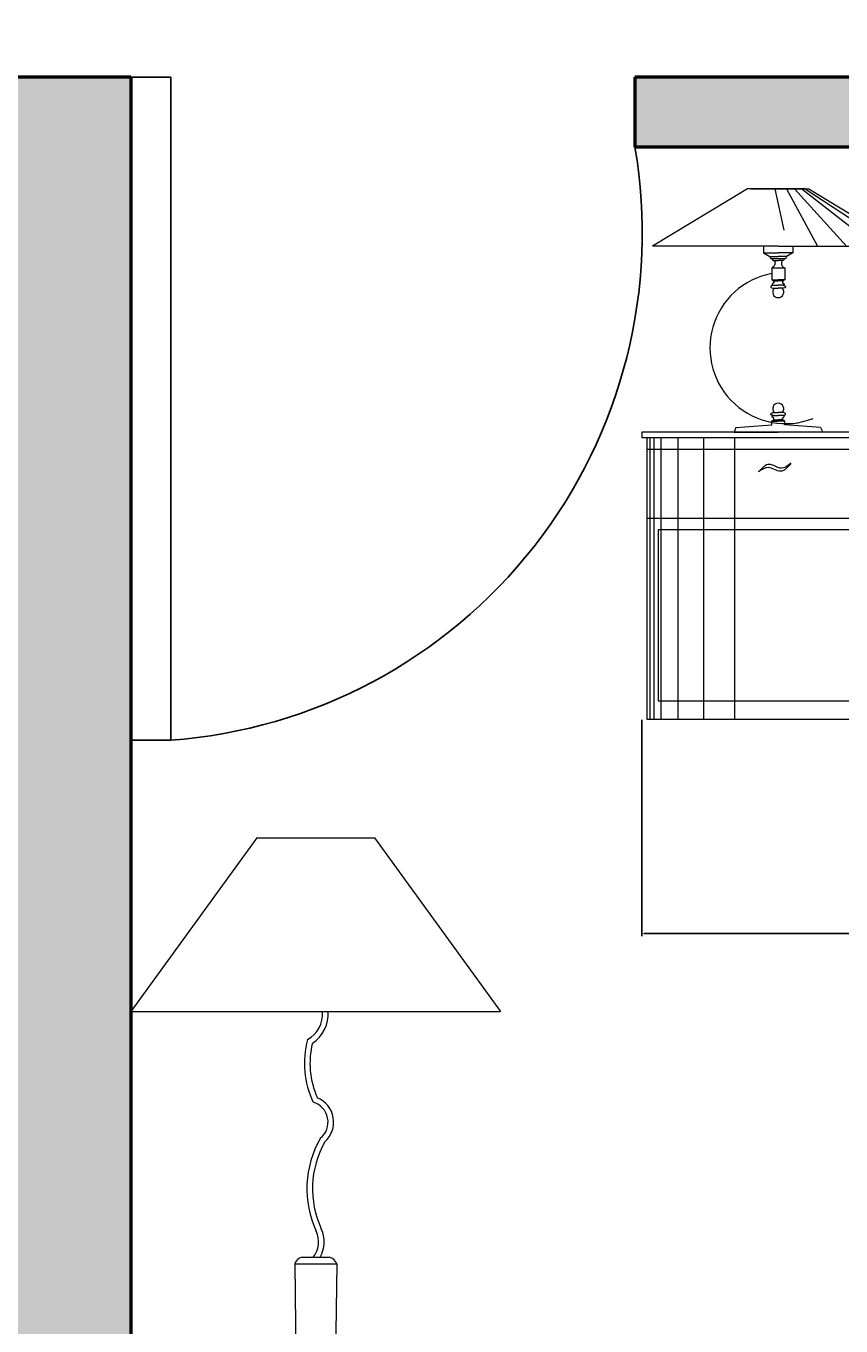
# Model space of a CAD drawing. Units: inches. Extents: x 1771 to 3025, y 319 to 889.
# Tile 3 of 35: x 1939 to 1997, y 527 to 620. Entities that reach past the tile are written whole.
import ezdxf

# ---------------------------------------------------------------- set-up
doc = ezdxf.new("R2010")
doc.units = ezdxf.units.IN
doc.header["$MEASUREMENT"] = 0
for name, color, linetype, lineweight in [('A-ANNO-DIMS', 2, 'Continuous', 18), ('A-DOOR', 4, 'Continuous', 25), ('A-FURN', 8, 'Continuous', 18), ('A-WALL', 7, 'Continuous', 50), ('A-WALL-PATT', 254, 'Continuous', 13)]:
    doc.layers.add(name, color=color, linetype=linetype, lineweight=lineweight)
doc.styles.get("Standard").update_dxf_attribs({"font": 'arial.ttf'})
doc.dimstyles.get("Standard").update_dxf_attribs({"dimtxt": 0.18, "dimasz": 0.18, "dimexe": 0.18, "dimexo": 0.0625, "dimgap": 0.09, "dimtad": 0, "dimtih": 1, "dimtoh": 1, "dimdec": 4, "dimzin": 0, "dimdsep": 46, "dimtxsty": 'Standard', "dimcen": 0.09, "dimadec": 0, "dimazin": 0, "dimtfac": 1, "dimtdec": 4, "dimtofl": 0, "dimtmove": 0, "dimatfit": 3, "dimfxl": 1, "dimtolj": 1, "dimtzin": 0, "dimarcsym": 0})

# ---------------------------------------------------------------- blocks, each defined once
blk = doc.blocks.new('A$C3908634B')
for p, q in [((184.3, 923.4), (19, 823.1)), ((237.5, 923.4), (184.3, 923.4)), ((190.2, 923.4), (237.5, 923.4)), ((231.9, 923.4), (247.3, 851.1)), ((284.7, 923.4), (237.5, 923.4)), ((237.5, 923.4), (290.6, 923.4)), ((251.7, 923.4), (305.7, 823.1)), ((266, 923.4), (356.4, 823.1)), ((278.7, 923.4), (406.8, 823.1)), ((284.7, 923.4), (436.3, 823.1)), ((290.6, 923.4), (456, 823.1)), ((237.5, 823.1), (19, 823.1)), ((212, 823.1), (212, 811.7)), ((237.5, 823.1), (456, 823.1)), ((263, 823.1), (263, 811.7)), ((212, 811.7), (223, 805.4)), ((212, 811.7), (237.5, 811.7)), ((223, 805.4), (224.6, 801.4)), ((223, 805.4), (237.5, 805.4)), ((250.4, 801.4), (224.6, 801.4)), ((226.9, 801.4), (228.3, 798.3)), ((228.3, 798.3), (237.5, 798.3)), ((228.3, 798.3), (231.3, 797.6)), ((231.3, 797.6), (232, 794.9)), ((231.6, 792.6), (231.5, 791.9)), ((231.9, 793.9), (231.6, 792.6)), ((232, 794.9), (231.9, 793.9)), ((263, 811.7), (237.5, 811.7)), ((252, 805.4), (237.5, 805.4)), ((246.7, 798.3), (237.5, 798.3)), ((243.7, 797.6), (243, 794.9)), ((243, 794.9), (243.1, 793.9)), ((243.1, 793.9), (243.4, 792.6)), ((243.4, 792.6), (243.4, 791.9)), ((246.7, 798.3), (243.7, 797.6)), ((248.1, 801.4), (246.7, 798.3)), ((252, 805.4), (250.4, 801.4)), ((263, 811.7), (252, 805.4)), ((227.8, 786.4), (226.2, 785.6)), ((226.2, 785.6), (226.2, 765)), ((226.2, 785.6), (248.8, 785.6)), ((230.2, 788), (227.8, 786.4)), ((231.1, 790.5), (230.2, 788)), ((231.5, 791.1), (231.1, 790.5)), ((231.5, 791.9), (231.5, 791.1)), ((243.4, 791.9), (243.4, 791.1)), ((243.4, 791.1), (243.9, 790.5)), ((243.9, 790.5), (244.8, 788)), ((244.8, 788), (247.2, 786.4)), ((247.2, 786.4), (248.8, 785.6)), ((248.8, 785.6), (248.8, 765)), ((224.8, 753.5), (224.7, 752.9)), ((224.7, 752.9), (224.8, 752.1)), ((225.3, 753.9), (224.8, 753.5)), ((224.8, 752.1), (225.2, 751.4)), ((225.2, 751.4), (225.6, 750.9)), ((225.7, 754.3), (225.3, 753.9)), ((225.6, 750.9), (228.1, 750.2)), ((226.3, 754.6), (225.7, 754.3)), ((226.2, 765), (227.6, 764.2)), ((226.2, 765), (237.5, 765)), ((227, 754.7), (226.3, 754.6)), ((227.9, 754.7), (227, 754.7)), ((227.4, 757.9), (227.1, 757.2)), ((227.1, 757.2), (227.3, 756.6)), ((227.3, 756.6), (227.8, 755.9)), ((227.7, 758.5), (227.4, 757.9)), ((227.6, 764.2), (228.5, 763.3)), ((228.6, 758.7), (227.7, 758.5)), ((227.8, 755.9), (228.9, 755.2)), ((228.9, 755.2), (227.9, 754.7)), ((228.1, 750.2), (229.9, 750)), ((228.5, 763.3), (229.4, 762.5)), ((228.5, 763.3), (237.5, 763.3)), ((229.4, 759.1), (228.6, 758.7)), ((228.9, 755.2), (237.5, 755.2)), ((229.4, 762.5), (230, 761.4)), ((229.8, 759.5), (229.4, 759.1)), ((230.1, 760.2), (229.8, 759.5)), ((229.9, 750), (232.4, 750.2)), ((230, 761.4), (230.1, 760.2)), ((232.4, 750.2), (237.5, 750.2)), ((248.8, 765), (237.5, 765)), ((246.5, 763.3), (237.5, 763.3)), ((246.1, 755.2), (237.5, 755.2)), ((242.6, 750.2), (237.5, 750.2)), ((245.1, 750), (242.6, 750.2)), ((245, 761.4), (244.9, 760.2)), ((244.9, 760.2), (245.2, 759.5)), ((245.6, 762.5), (245, 761.4)), ((246.9, 750.2), (245.1, 750)), ((245.2, 759.5), (245.6, 759.1)), ((246.5, 763.3), (245.6, 762.5)), ((245.6, 759.1), (246.4, 758.7)), ((247.2, 755.9), (246.1, 755.2)), ((246.1, 755.2), (247.1, 754.7)), ((246.4, 758.7), (247.3, 758.5)), ((247.4, 764.2), (246.5, 763.3)), ((249.4, 750.9), (246.9, 750.2)), ((247.1, 754.7), (248, 754.7)), ((247.7, 756.6), (247.2, 755.9)), ((247.3, 758.5), (247.6, 757.9)), ((248.8, 765), (247.4, 764.2)), ((247.6, 757.9), (247.9, 757.2)), ((247.9, 757.2), (247.7, 756.6)), ((248, 754.7), (248.7, 754.6)), ((248.7, 754.6), (249.3, 754.3)), ((249.3, 754.3), (249.7, 753.9)), ((249.8, 751.4), (249.4, 750.9)), ((249.7, 753.9), (250.2, 753.5)), ((250.2, 752.1), (249.8, 751.4)), ((250.2, 753.5), (250.3, 752.9)), ((250.3, 752.9), (250.2, 752.1)), ((224.7, 530.9), (224.8, 531.7)), ((224.8, 530.3), (224.7, 530.9)), ((224.8, 531.7), (225.2, 532.4)), ((225.3, 529.9), (224.8, 530.3)), ((225.2, 532.4), (225.6, 532.9)), ((225.7, 529.5), (225.3, 529.9)), ((225.6, 532.9), (228.1, 533.6)), ((226.3, 529.2), (225.7, 529.5)), ((227, 529.1), (226.3, 529.2)), ((227.9, 529.1), (227, 529.1)), ((227.1, 526.6), (227.3, 527.2)), ((227.4, 525.9), (227.1, 526.6)), ((227.3, 527.2), (227.8, 527.9)), ((227.7, 525.3), (227.4, 525.9)), ((228.6, 525.1), (227.7, 525.3)), ((227.8, 527.9), (228.9, 528.6)), ((228.9, 528.6), (227.9, 529.1)), ((228.1, 533.6), (229.9, 533.8)), ((228.5, 520.5), (229.4, 521.3)), ((229.4, 524.7), (228.6, 525.1)), ((228.9, 528.6), (237.5, 528.6)), ((229.8, 524.3), (229.4, 524.7)), ((229.4, 521.3), (230, 522.4)), ((229.4, 521.3), (237.5, 521.3)), ((230.1, 523.6), (229.8, 524.3)), ((230, 522.4), (230.1, 523.6)), ((230.3, 533.8), (237.5, 533.6)), ((242.6, 533.6), (237.5, 533.6)), ((246.1, 528.6), (237.5, 528.6)), ((245.6, 521.3), (237.5, 521.3)), ((245.1, 533.8), (242.6, 533.6)), ((244.9, 523.6), (245.2, 524.3)), ((245, 522.4), (244.9, 523.6)), ((245.6, 521.3), (245, 522.4)), ((246.9, 533.6), (245.1, 533.8)), ((245.2, 524.3), (245.6, 524.7)), ((245.6, 524.7), (246.4, 525.1)), ((246.5, 520.5), (245.6, 521.3)), ((246.1, 528.6), (247.1, 529.1)), ((247.2, 527.9), (246.1, 528.6)), ((246.4, 525.1), (247.3, 525.3)), ((249.4, 532.9), (246.9, 533.6)), ((247.1, 529.1), (248, 529.1)), ((247.7, 527.2), (247.2, 527.9)), ((247.3, 525.3), (247.6, 525.9)), ((247.6, 525.9), (247.9, 526.6)), ((247.9, 526.6), (247.7, 527.2)), ((248, 529.1), (248.7, 529.2)), ((248.7, 529.2), (249.3, 529.5)), ((249.3, 529.5), (249.7, 529.9)), ((249.8, 532.4), (249.4, 532.9)), ((249.7, 529.9), (250.2, 530.3)), ((250.2, 531.7), (249.8, 532.4)), ((250.3, 530.9), (250.2, 531.7)), ((250.2, 530.3), (250.3, 530.9)), ((475, 499.5), (0, 499.5)), ((0, 499.5), (0, 489.5)), ((164, 507.9), (161.1, 499.5)), ((161.1, 499.5), (237.5, 499.5)), ((164, 507.9), (226.2, 512.1)), ((226.2, 518.8), (227.6, 519.6)), ((226.2, 512.1), (226.2, 518.8)), ((226.2, 518.8), (237.5, 518.8)), ((227.6, 519.6), (228.5, 520.5)), ((248.8, 518.8), (237.5, 518.8)), ((315.3, 499.5), (237.5, 499.5)), ((247.4, 519.6), (246.5, 520.5)), ((248.8, 518.8), (247.4, 519.6)), ((248.8, 512.1), (248.8, 518.8)), ((311, 507.9), (248.8, 512.1)), ((311, 507.9), (315.3, 499.5)), ((475, 489.5), (0, 489.5)), ((8.7, 489.5), (8.7, 0)), ((14.1, 488.6), (14.1, 0)), ((21.3, 488.6), (21.3, 0)), ((33, 488.6), (33, 0)), ((62.7, 488.6), (62.7, 0)), ((107.6, 488.6), (107.6, 0)), ((161.6, 488.6), (161.6, 0)), ((467.1, 469.5), (8.7, 469.5)), ((467.1, 349.5), (8.7, 349.5)), ((28.7, 329.5), (28.7, 31.6)), ((447.1, 329.5), (28.7, 329.5)), ((28.7, 31.6), (447.1, 31.6)), ((8.7, 0), (467.1, 0))]:
    blk.add_line(p, q)
for centre, radius, start, end in [((250.5, 646.2), 131.8, 100.6234, 291.2), ((237.5, 743.5), 9.69, 137.7341, 270), ((237.5, 743.5), 9.69, 270, 42.2659), ((237.5, 540.3), 9.69, 90, 222.2659), ((237.5, 540.3), 9.69, 317.7341, 90)]:
    blk.add_arc(centre, radius, start, end)
for points, knots in [([(259.6, 445.5), (254.3, 441.1), (244.8, 433.2), (231.9, 440.9), (217, 446), (209.2, 437.1), (203.4, 430.5)], [0, 0, 0, 0, 18.381528, 32.980054, 40.875646, 63.595153, 63.595153, 63.595153, 63.595153]), ([(259.6, 445.5), (254, 438.6), (242.8, 424.9), (221, 442.9), (208.9, 434.4), (203.4, 430.5)], [0, 0, 0, 0, 22.772447, 45.052082, 63.466582, 63.466582, 63.466582, 63.466582])]:
    blk.add_open_spline(points, degree=3, knots=knots)
blk = doc.blocks.new('A$C0DCF6C46')
for p, q in [((179.4, 1650), (0, 1402.3)), ((179.4, 1650), (0, 1402.3)), ((179.4, 1650), (347.3, 1650)), ((179.4, 1650), (347.3, 1650)), ((347.3, 1650), (526.7, 1402.3)), ((347.3, 1650), (526.7, 1402.3)), ((0, 1402.3), (526.7, 1402.3)), ((0, 1402.3), (526.7, 1402.3)), ((1227.6, 1090.4), (1251, 1095.4)), ((1227.6, 1090.4), (1251, 1095.4)), ((1251, 1095.4), (1277.5, 1092)), ((1251, 1095.4), (1277.5, 1092)), ((1202.6, 1072.4), (1213.4, 1083.3)), ((1202.6, 1072.4), (1213.4, 1083.3)), ((1213.4, 1083.3), (1227.6, 1090.4)), ((1213.4, 1083.3), (1227.6, 1090.4)), ((1277.5, 1092), (1301.8, 1082.8)), ((1277.5, 1092), (1301.8, 1082.8)), ((1301.8, 1082.8), (1321.9, 1067.8)), ((1301.8, 1082.8), (1321.9, 1067.8)), ((1173.6, 1032.9), (1189.7, 1057.2)), ((1173.6, 1032.9), (1189.7, 1057.2)), ((1189.7, 1057.2), (1202.6, 1072.4)), ((1189.7, 1057.2), (1202.6, 1072.4)), ((1259.7, 1050.3), (1237.5, 1065.3)), ((1259.7, 1050.3), (1237.5, 1065.3)), ((1321.9, 1067.8), (1345.5, 1041.1)), ((1321.9, 1067.8), (1345.5, 1041.1)), ((233.4, 1042.3), (293.3, 1042.3)), ((233.4, 1042.3), (235.7, 853.7)), ((233.4, 1042.3), (293.3, 1042.3)), ((233.4, 1042.3), (235.7, 853.7)), ((244, 1051.7), (282.6, 1051.7)), ((244, 1051.7), (282.6, 1051.7)), ((293.3, 1042.3), (290.8, 843.9)), ((293.3, 1042.3), (290.8, 843.9)), ((1255.9, 1046.6), (1245.7, 1027.6)), ((1255.9, 1046.6), (1245.7, 1027.6)), ((1278.7, 1041.6), (1259.7, 1050.3)), ((1278.7, 1041.6), (1259.7, 1050.3)), ((1308.3, 1028.1), (1278.7, 1041.6)), ((1308.3, 1028.1), (1278.7, 1041.6)), ((1345.5, 1041.1), (1350.1, 1013.5)), ((1345.5, 1041.1), (1350.1, 1013.5)), ((1150.8, 970.5), (1173.6, 1032.9)), ((1150.8, 970.5), (1173.6, 1032.9)), ((1245.7, 1027.6), (1232.3, 1009.1)), ((1245.7, 1027.6), (1232.3, 1009.1)), ((1335.8, 1012.5), (1308.3, 1028.1)), ((1335.8, 1012.5), (1308.3, 1028.1)), ((1232.3, 1009.1), (1218.3, 983.7)), ((1232.3, 1009.1), (1218.3, 983.7)), ((1338.8, 997.1), (1335.8, 1012.5)), ((1338.8, 997.1), (1335.8, 1012.5)), ((1350.1, 1013.5), (1354.2, 991.7)), ((1350.1, 1013.5), (1354.2, 991.7)), ((1190.8, 987.7), (1188, 972.3)), ((1190.8, 987.7), (1188, 972.3)), ((1202.9, 975.4), (1190.8, 987.7)), ((1202.9, 975.4), (1190.8, 987.7)), ((1218.3, 983.7), (1202.9, 975.4)), ((1218.3, 983.7), (1202.9, 975.4)), ((1277.8, 994.4), (1265.6, 995)), ((1277.8, 994.4), (1265.6, 995)), ((1291.5, 983.2), (1277.8, 994.4)), ((1291.5, 983.2), (1277.8, 994.4)), ((1354.2, 991.7), (1333.4, 980.2)), ((1354.2, 991.7), (1333.4, 980.2)), ((1334, 990.3), (1338.8, 997.1)), ((1334, 990.3), (1338.8, 997.1)), ((1147.4, 942.9), (1150.8, 970.5)), ((1147.4, 942.9), (1150.8, 970.5)), ((1188, 972.3), (1182.6, 958)), ((1188, 972.3), (1182.6, 958)), ((1266, 980.7), (1284.6, 977.9)), ((1266, 980.7), (1284.6, 977.9)), ((1304.1, 966.6), (1297.6, 940.6)), ((1304.1, 966.6), (1297.6, 940.6)), ((1309.5, 977.7), (1304.1, 966.6)), ((1309.5, 977.7), (1304.1, 966.6)), ((1309.4, 969), (1312.6, 964.7)), ((1314.7, 968.9), (1309.4, 969)), ((1309.4, 969), (1312.6, 964.7)), ((1314.7, 968.9), (1309.4, 969)), ((1317.5, 977.7), (1309.5, 977.7)), ((1317.5, 977.7), (1309.5, 977.7)), ((1324.9, 973.9), (1322.1, 963.3)), ((1324.9, 973.9), (1322.1, 963.3)), ((1333.4, 980.2), (1324.9, 973.9)), ((1333.4, 980.2), (1324.9, 973.9)), ((1318.8, 948.5), (1307.6, 932.1)), ((1318.8, 948.5), (1307.6, 932.1)), ((1322.1, 963.3), (1318.8, 948.5)), ((1322.1, 963.3), (1318.8, 948.5)), ((1087.8, 908.4), (1135.7, 928.2)), ((1087.8, 908.4), (1135.7, 928.2)), ((1135.7, 928.2), (1147.4, 942.9)), ((1135.7, 928.2), (1147.4, 942.9)), ((1170.4, 917.1), (1156.8, 933.1)), ((1170.4, 917.1), (1156.8, 933.1)), ((1307.6, 932.1), (1282.5, 914.8)), ((1307.6, 932.1), (1282.5, 914.8)), ((1297.6, 940.6), (1286.8, 941.4)), ((1297.6, 940.6), (1286.8, 941.4)), ((1117, 920.9), (1113.7, 907.1)), ((1117, 920.9), (1113.7, 907.1)), ((1190.9, 864.1), (1144, 915.9)), ((1190.9, 864.1), (1144, 915.9)), ((1211.2, 886.7), (1170.4, 917.1)), ((1211.2, 886.7), (1170.4, 917.1)), ((1225.9, 897.6), (1208.3, 912.3)), ((1225.9, 897.6), (1208.3, 912.3)), ((1282.5, 914.8), (1267, 899.5)), ((1282.5, 914.8), (1267, 899.5)), ((1295.1, 904.1), (1310, 911.9)), ((1295.1, 904.1), (1310, 911.9)), ((1310, 911.9), (1334.4, 909.6)), ((1310, 911.9), (1334.4, 909.6)), ((1334.4, 909.6), (1359.2, 894.6)), ((1334.4, 909.6), (1359.2, 894.6)), ((995.7, 868.8), (1011.8, 893.6)), ((995.7, 868.8), (1011.8, 893.6)), ((1011.8, 893.6), (1033.6, 897.7)), ((1011.8, 893.6), (1033.6, 897.7)), ((1033.6, 897.7), (1060.7, 904.4)), ((1033.6, 897.7), (1060.7, 904.4)), ((1039.9, 891.8), (1050.5, 891.7)), ((1039.9, 891.8), (1050.5, 891.7)), ((1050.5, 891.7), (1058.4, 882.1)), ((1050.5, 891.7), (1058.4, 882.1)), ((1060.7, 904.4), (1087.8, 908.4)), ((1060.7, 904.4), (1087.8, 908.4)), ((1113.7, 907.1), (1121.7, 900.7)), ((1113.7, 907.1), (1121.7, 900.7)), ((1121.7, 900.7), (1119.4, 884.3)), ((1121.7, 900.7), (1119.4, 884.3)), ((1240.6, 890.8), (1225.9, 897.6)), ((1240.6, 890.8), (1225.9, 897.6)), ((1254.3, 890.2), (1240.6, 890.8)), ((1254.3, 890.2), (1240.6, 890.8)), ((1264.4, 895.9), (1254.3, 890.2)), ((1264.4, 895.9), (1254.3, 890.2)), ((1267, 899.5), (1271.7, 895.8)), ((1267, 899.5), (1271.7, 895.8)), ((1271.7, 895.8), (1295.1, 904.1)), ((1271.7, 895.8), (1295.1, 904.1)), ((1359.2, 894.6), (1384, 866.8)), ((1359.2, 894.6), (1384, 866.8)), ((1058.4, 882.1), (1076.1, 842.2)), ((1058.4, 882.1), (1076.1, 842.2)), ((1119.4, 884.3), (1119.3, 867.8)), ((1119.4, 884.3), (1119.3, 867.8)), ((1211.2, 886.7), (1190.9, 864.1)), ((1211.2, 886.7), (1190.9, 864.1)), ((1222.8, 881.9), (1223.6, 853.9)), ((1247, 848.8), (1222.8, 881.9)), ((1222.8, 881.9), (1223.6, 853.9)), ((1247, 848.8), (1222.8, 881.9)), ((1303.8, 861.6), (1313.5, 875.8)), ((1303.8, 861.6), (1313.5, 875.8)), ((1313.5, 875.8), (1318.8, 876.9)), ((1313.5, 875.8), (1318.8, 876.9)), ((1318.8, 876.9), (1321.4, 867.3)), ((1318.8, 876.9), (1321.4, 867.3)), ((148.7, 869.2), (799.3, 753.3)), ((148.7, 869.2), (799.3, 753.3)), ((986.5, 846.6), (995.7, 868.8)), ((986.5, 846.6), (995.7, 868.8)), ((1119.3, 867.8), (1135.5, 846.5)), ((1119.3, 867.8), (1135.5, 846.5)), ((1186.6, 860.4), (1212.2, 811.9)), ((1186.6, 860.4), (1212.2, 811.9)), ((1196.7, 865.6), (1204.6, 855)), ((1196.7, 865.6), (1204.6, 855)), ((1204.6, 855), (1219.4, 853.2)), ((1204.6, 855), (1219.4, 853.2)), ((1223.6, 853.9), (1255.4, 801.3)), ((1223.6, 853.9), (1255.4, 801.3)), ((1275.8, 869.8), (1284.7, 863.3)), ((1275.8, 869.8), (1284.7, 863.3)), ((1278.8, 848), (1280, 865.5)), ((1278.8, 848), (1280, 865.5)), ((1284.7, 863.3), (1296.3, 854.2)), ((1284.7, 863.3), (1296.3, 854.2)), ((1296.3, 854.2), (1303.8, 861.6)), ((1296.3, 854.2), (1303.8, 861.6)), ((1321.4, 867.3), (1342.5, 854.4)), ((1321.4, 867.3), (1342.5, 854.4)), ((1342.5, 854.4), (1362, 845.8)), ((1342.5, 854.4), (1362, 845.8)), ((1384, 866.8), (1396.6, 853.4)), ((1384, 866.8), (1396.6, 853.4)), ((1396.6, 853.4), (1411.8, 831)), ((1396.6, 853.4), (1411.8, 831)), ((984.8, 829.6), (986.5, 846.6)), ((984.8, 829.6), (986.5, 846.6)), ((1076.1, 842.2), (1077.8, 785.9)), ((1076.1, 842.2), (1077.8, 785.9)), ((1135.5, 846.5), (1162.3, 812.3)), ((1135.5, 846.5), (1162.3, 812.3)), ((1213.6, 851.7), (1221.1, 799.1)), ((1213.6, 851.7), (1221.1, 799.1)), ((1257.2, 799.9), (1247, 848.8)), ((1257.2, 799.9), (1247, 848.8)), ((1293.6, 844.7), (1278.8, 848)), ((1293.6, 844.7), (1278.8, 848)), ((1293.9, 818.2), (1293.6, 844.7)), ((1293.9, 818.2), (1293.6, 844.7)), ((1325.9, 840.7), (1312.2, 852)), ((1325.9, 840.7), (1312.2, 852)), ((1343.2, 816.2), (1325.9, 840.7)), ((1343.2, 816.2), (1325.9, 840.7)), ((1362, 845.8), (1365, 822.9)), ((1362, 845.8), (1365, 822.9)), ((1637.6, 846.8), (1643.1, 837.5)), ((1637.6, 846.8), (1643.1, 837.5)), ((1680.1, 723.7), (1660.3, 834.6)), ((1680.1, 723.7), (1660.3, 834.6)), ((915.2, 833), (897.4, 738.2)), ((915.2, 833), (897.4, 738.2)), ((970.2, 796.3), (984.8, 829.6)), ((970.2, 796.3), (984.8, 829.6)), ((1296.3, 781), (1293.9, 818.2)), ((1296.3, 781), (1293.9, 818.2)), ((1364.9, 799.6), (1343.2, 816.2)), ((1364.9, 799.6), (1343.2, 816.2)), ((1376.2, 822.8), (1365, 822.9)), ((1365, 822.9), (1371.3, 804.3)), ((1376.2, 822.8), (1365, 822.9)), ((1365, 822.9), (1371.3, 804.3)), ((1390.5, 825.9), (1376.2, 822.8)), ((1390.5, 825.9), (1376.2, 822.8)), ((1401.2, 832.2), (1390.5, 825.9)), ((1401.2, 832.2), (1390.5, 825.9)), ((1405.2, 808.3), (1401.2, 832.2)), ((1405.2, 808.3), (1401.2, 832.2)), ((1411.8, 831), (1422.3, 818.2)), ((1411.8, 831), (1422.3, 818.2)), ((1414.4, 832.1), (1447.5, 790.5)), ((1414.4, 832.1), (1447.5, 790.5)), ((1422.3, 818.2), (1423.8, 807.1)), ((1422.3, 818.2), (1423.8, 807.1)), ((167.7, 0), (90.2, 815.3)), ((167.7, 0), (90.2, 815.3)), ((1162.3, 812.3), (1187.5, 779.8)), ((1162.3, 812.3), (1187.5, 779.8)), ((1212.2, 811.9), (1236.7, 763.5)), ((1212.2, 811.9), (1236.7, 763.5)), ((1275.4, 760.5), (1257.2, 799.9)), ((1275.4, 760.5), (1257.2, 799.9)), ((1371.3, 804.3), (1380.5, 770.8)), ((1371.3, 804.3), (1380.5, 770.8)), ((1384, 803.7), (1372.4, 811.7)), ((1384, 803.7), (1372.4, 811.7)), ((1403.6, 803.5), (1384, 803.7)), ((1403.6, 803.5), (1384, 803.7)), ((1423.8, 807.1), (1403.6, 803.5)), ((1423.8, 807.1), (1403.6, 803.5)), ((1431.7, 801.7), (1440.8, 748.6)), ((1431.7, 801.7), (1440.8, 748.6)), ((821.8, 697.8), (222.3, 796.3)), ((821.8, 697.8), (222.3, 796.3)), ((966.3, 773.5), (970.2, 796.3)), ((966.3, 773.5), (970.2, 796.3)), ((1077.8, 785.9), (1071.1, 747.3)), ((1077.8, 785.9), (1071.1, 747.3)), ((1187.5, 779.8), (1212.2, 747.2)), ((1187.5, 779.8), (1212.2, 747.2)), ((1304.4, 731.6), (1296.3, 781)), ((1304.4, 731.6), (1296.3, 781)), ((1447.5, 790.5), (1463.6, 748.4)), ((1447.5, 790.5), (1463.6, 748.4)), ((963, 758.2), (966.3, 773.5)), ((963, 758.2), (966.3, 773.5)), ((1236.7, 763.5), (1253.3, 709.8)), ((1236.7, 763.5), (1253.3, 709.8)), ((1294.7, 714.7), (1275.4, 760.5)), ((1294.7, 714.7), (1275.4, 760.5)), ((1380.5, 770.8), (1387.2, 743.7)), ((1380.5, 770.8), (1387.2, 743.7)), ((965.8, 711), (963, 758.2)), ((965.8, 711), (963, 758.2)), ((1071.1, 747.3), (1070.3, 709.1)), ((1071.1, 747.3), (1070.3, 709.1)), ((1212.2, 747.2), (1239, 712)), ((1212.2, 747.2), (1239, 712)), ((1387.2, 743.7), (1387.1, 723)), ((1387.2, 743.7), (1387.1, 723)), ((1463.6, 748.4), (1467.1, 713.4)), ((1463.6, 748.4), (1467.1, 713.4)), ((816.5, 736.2), (823.2, 687.2)), ((816.5, 736.2), (823.2, 687.2)), ((1310.9, 687.6), (1304.4, 731.6)), ((1310.9, 687.6), (1304.4, 731.6)), ((949, 665.5), (965.8, 711)), ((949, 665.5), (965.8, 711)), ((1070.3, 709.1), (1067.4, 681)), ((1070.3, 709.1), (1067.4, 681)), ((1239, 712), (1250, 700.8)), ((1239, 712), (1250, 700.8)), ((1253.3, 709.8), (1262, 665.7)), ((1253.3, 709.8), (1262, 665.7)), ((1319.7, 657.3), (1294.7, 714.7)), ((1319.7, 657.3), (1294.7, 714.7)), ((1387.1, 723), (1385.3, 706.1)), ((1387.1, 723), (1385.3, 706.1)), ((1410.2, 693.1), (1433.6, 709.9)), ((1410.2, 693.1), (1433.6, 709.9)), ((1433.6, 709.9), (1459.6, 709.7)), ((1433.6, 709.9), (1459.6, 709.7)), ((1467.1, 713.4), (1510.5, 701.4)), ((1467.1, 713.4), (1510.5, 701.4)), ((823.2, 687.2), (840.7, 645.7)), ((823.2, 687.2), (840.7, 645.7)), ((919.8, 701.9), (919.8, 0)), ((919.8, 701.9), (919.8, 0)), ((1325.9, 701.8), (1321.2, 649.3)), ((1325.9, 701.8), (1321.2, 649.3)), ((1387.8, 675.8), (1325.9, 701.8)), ((1387.8, 675.8), (1325.9, 701.8)), ((1387.8, 675.8), (1410.2, 693.1)), ((1387.8, 675.8), (1410.2, 693.1)), ((1510.5, 701.4), (1562.3, 673.9)), ((1510.5, 701.4), (1562.3, 673.9)), ((1656.8, 701.9), (1656.8, 607.1)), ((1656.8, 701.9), (1656.8, 607.1)), ((816.1, 675.1), (831.6, 638.4)), ((816.1, 675.1), (831.6, 638.4)), ((968.1, 667.4), (995.8, 675.7)), ((968.1, 667.4), (995.8, 675.7)), ((995.8, 675.7), (1036.1, 673.3)), ((995.8, 675.7), (1036.1, 673.3)), ((1036.1, 673.3), (1074.2, 672.4)), ((1036.1, 673.3), (1074.2, 672.4)), ((1074.2, 672.4), (1099.7, 668.5)), ((1074.2, 672.4), (1099.7, 668.5)), ((1099.7, 668.5), (1130.9, 665.6)), ((1099.7, 668.5), (1130.9, 665.6)), ((1362.7, 657.4), (1387.8, 675.8)), ((1362.7, 657.4), (1387.8, 675.8)), ((1562.3, 673.9), (1616.6, 642.7)), ((1562.3, 673.9), (1616.6, 642.7)), ((952.4, 624.6), (949, 665.5)), ((952.4, 624.6), (949, 665.5)), ((1130.3, 647.1), (1138.8, 656.6)), ((1130.3, 647.1), (1138.8, 656.6)), ((1130.9, 665.6), (1156.4, 659.6)), ((1130.9, 665.6), (1156.4, 659.6)), ((1156.4, 659.6), (1194, 656.7)), ((1156.4, 659.6), (1194, 656.7)), ((1194, 656.7), (1230, 653.7)), ((1194, 656.7), (1230, 653.7)), ((1230, 653.7), (1248, 637.7)), ((1230, 653.7), (1248, 637.7)), ((1262, 665.7), (1274.2, 603)), ((1262, 665.7), (1274.2, 603)), ((1321.2, 649.3), (1340.1, 623.1)), ((1321.2, 649.3), (1340.1, 623.1)), ((1342.9, 632.7), (1362.7, 657.4)), ((1342.9, 632.7), (1362.7, 657.4)), ((1569.5, 644.7), (1548.9, 662.4)), ((1569.5, 644.7), (1548.9, 662.4)), ((831.6, 638.4), (853.4, 612.1)), ((831.6, 638.4), (853.4, 612.1)), ((840.7, 645.7), (862.6, 619.4)), ((840.7, 645.7), (862.6, 619.4)), ((1120.6, 625.4), (1130.3, 647.1)), ((1120.6, 625.4), (1130.3, 647.1)), ((1248, 637.7), (1261.6, 613.2)), ((1248, 637.7), (1261.6, 613.2)), ((1325.7, 613.7), (1342.9, 632.7)), ((1325.7, 613.7), (1342.9, 632.7)), ((1361.5, 647.4), (1329.7, 647.6)), ((1361.5, 647.4), (1329.7, 647.6)), ((1595.2, 618), (1569.5, 644.7)), ((1595.2, 618), (1569.5, 644.7)), ((1616.6, 642.7), (1655.6, 607.9)), ((1616.6, 642.7), (1655.6, 607.9)), ((853.4, 612.1), (858.7, 592.9)), ((853.4, 612.1), (858.7, 592.9)), ((862.6, 619.4), (867.8, 600.3)), ((862.6, 619.4), (867.8, 600.3)), ((961.2, 603.3), (952.4, 624.6)), ((961.2, 603.3), (952.4, 624.6)), ((1119.9, 607.9), (1120.6, 625.4)), ((1119.9, 607.9), (1120.6, 625.4)), ((1261.6, 613.2), (1259.1, 569.7)), ((1261.6, 613.2), (1259.1, 569.7)), ((1304.9, 592.7), (1325.7, 613.7)), ((1304.9, 592.7), (1325.7, 613.7)), ((1503.4, 603.8), (1505.1, 628.7)), ((1503.4, 603.8), (1505.1, 628.7)), ((1618.8, 582.8), (1595.2, 618)), ((1618.8, 582.8), (1595.2, 618)), ((867.8, 600.3), (810.7, 0)), ((867.8, 600.3), (810.7, 0)), ((994.1, 595.1), (961.2, 603.3)), ((994.1, 595.1), (961.2, 603.3)), ((1053.9, 576.6), (994.1, 595.1)), ((1053.9, 576.6), (994.1, 595.1)), ((1111.3, 595.2), (1113.2, 565.5)), ((1111.3, 595.2), (1113.2, 565.5)), ((1115.1, 607.9), (1115, 596.8)), ((1115.1, 607.9), (1115, 596.8)), ((1128.9, 611.5), (1115.1, 607.9)), ((1128.9, 611.5), (1115.1, 607.9)), ((1115.6, 599.4), (1119.9, 607.9)), ((1115.6, 599.4), (1119.9, 607.9)), ((1154.9, 605), (1128.9, 611.5)), ((1154.9, 605), (1128.9, 611.5)), ((1202.6, 606.7), (1154.9, 605)), ((1202.6, 606.7), (1154.9, 605)), ((1217.8, 581.7), (1202.6, 606.7)), ((1217.8, 581.7), (1202.6, 606.7)), ((1274.2, 603), (1280.6, 545.6)), ((1274.2, 603), (1280.6, 545.6)), ((1475.8, 608.8), (1478.2, 578)), ((1491.8, 546.1), (1475.8, 608.8)), ((1475.8, 608.8), (1478.2, 578)), ((1491.8, 546.1), (1475.8, 608.8)), ((1501, 578.9), (1503.4, 603.8)), ((1501, 578.9), (1503.4, 603.8)), ((1655.6, 607.9), (1695.2, 580.6)), ((1655.6, 607.9), (1695.2, 580.6)), ((858.7, 592.9), (816.6, 146.6)), ((858.7, 592.9), (816.6, 146.6)), ((1112.1, 561.3), (1053.9, 576.6)), ((1112.1, 561.3), (1053.9, 576.6)), ((1228.9, 581.6), (1217.8, 581.7)), ((1228.9, 581.6), (1217.8, 581.7)), ((1228.2, 558.8), (1228.9, 581.6)), ((1228.2, 558.8), (1228.9, 581.6)), ((1284.6, 575.8), (1304.9, 592.7)), ((1284.6, 575.8), (1304.9, 592.7)), ((1478.2, 578), (1493.9, 543.4)), ((1478.2, 578), (1493.9, 543.4)), ((1489.2, 562.6), (1501, 578.9)), ((1489.2, 562.6), (1501, 578.9)), ((1635.5, 547.1), (1618.8, 582.8)), ((1635.5, 547.1), (1618.8, 582.8)), ((1695.2, 580.6), (1732.1, 555.4)), ((1695.2, 580.6), (1732.1, 555.4)), ((1128.3, 528.3), (1112.1, 561.3)), ((1128.3, 528.3), (1112.1, 561.3)), ((1252.7, 566), (1228.2, 558.8)), ((1252.7, 566), (1228.2, 558.8)), ((1259.1, 569.7), (1252.7, 566)), ((1259.1, 569.7), (1252.7, 566)), ((1280.6, 545.6), (1294.5, 479.8)), ((1280.6, 545.6), (1294.5, 479.8)), ((1478.3, 517.6), (1491.8, 546.1)), ((1478.3, 517.6), (1491.8, 546.1)), ((1493.9, 543.4), (1527.3, 540.5)), ((1493.9, 543.4), (1527.3, 540.5)), ((1527.3, 540.5), (1578.2, 538)), ((1527.3, 540.5), (1578.2, 538)), ((1578.2, 538), (1610.5, 537.7)), ((1578.2, 538), (1610.5, 537.7)), ((1732.1, 555.4), (1753.8, 546.2)), ((1732.1, 555.4), (1753.8, 546.2)), ((1747.8, 525.5), (1746.4, 548.4)), ((1747.8, 525.5), (1746.4, 548.4)), ((1753.8, 546.2), (1776.6, 543.9)), ((1753.8, 546.2), (1776.6, 543.9)), ((1776.6, 543.9), (1784.6, 547)), ((1776.6, 543.9), (1784.6, 547)), ((1788.3, 543.8), (1777, 533.3)), ((1788.3, 543.8), (1777, 533.3)), ((1784.6, 547), (1807.3, 541.5)), ((1784.6, 547), (1807.3, 541.5)), ((1807.3, 541.5), (1836.4, 528.5)), ((1807.3, 541.5), (1836.4, 528.5)), ((1142.4, 502.7), (1128.3, 528.3)), ((1142.4, 502.7), (1128.3, 528.3)), ((1610.5, 537.7), (1634.4, 534.9)), ((1610.5, 537.7), (1634.4, 534.9)), ((1634.4, 534.9), (1652.2, 511.4)), ((1634.4, 534.9), (1652.2, 511.4)), ((1747.1, 502.7), (1747.8, 525.5)), ((1747.1, 502.7), (1747.8, 525.5)), ((1777, 522.1), (1776.8, 504.6)), ((1777, 522.1), (1776.8, 504.6)), ((1777, 533.3), (1777, 522.1)), ((1777, 533.3), (1777, 522.1)), ((1836.4, 528.5), (1857.6, 518.8)), ((1836.4, 528.5), (1857.6, 518.8)), ((1162.3, 464.9), (1142.4, 502.7)), ((1162.3, 464.9), (1142.4, 502.7)), ((1447.7, 477), (1460.7, 501.8)), ((1447.7, 477), (1460.7, 501.8)), ((1460.7, 501.8), (1478.3, 517.6)), ((1460.7, 501.8), (1478.3, 517.6)), ((1556.5, 478.8), (1575.3, 505.7)), ((1556.5, 478.8), (1575.3, 505.7)), ((1652.2, 511.4), (1671, 474.2)), ((1652.2, 511.4), (1671, 474.2)), ((1740, 481), (1747.1, 502.7)), ((1740, 481), (1747.1, 502.7)), ((1776.8, 504.6), (1766.2, 498.3)), ((1776.8, 504.6), (1766.2, 498.3)), ((1857.6, 518.8), (1884.1, 516)), ((1857.6, 518.8), (1884.1, 516)), ((1884.1, 516), (1912.1, 507.8)), ((1884.1, 516), (1912.1, 507.8)), ((1912.1, 507.8), (1913, 492.4)), ((1912.1, 507.8), (1913, 492.4)), ((1766.2, 498.3), (1749.2, 494.8)), ((1766.2, 498.3), (1749.2, 494.8)), ((1913, 492.4), (1906, 476.6)), ((1913, 492.4), (1906, 476.6)), ((1170.5, 433.5), (1162.3, 464.9)), ((1170.5, 433.5), (1162.3, 464.9)), ((1294.5, 479.8), (1303.6, 427.7)), ((1294.5, 479.8), (1303.6, 427.7)), ((1415.7, 451.8), (1447.7, 477)), ((1415.7, 451.8), (1447.7, 477)), ((1547.8, 455), (1556.5, 478.8)), ((1547.8, 455), (1556.5, 478.8)), ((1671, 474.2), (1681.4, 448.6)), ((1671, 474.2), (1681.4, 448.6)), ((1732.4, 458.3), (1740, 481)), ((1732.4, 458.3), (1740, 481)), ((1906, 476.6), (1884.1, 456)), ((1906, 476.6), (1884.1, 456)), ((1379, 432.4), (1415.7, 451.8)), ((1379, 432.4), (1415.7, 451.8)), ((1546.6, 431.1), (1547.8, 455)), ((1546.6, 431.1), (1547.8, 455)), ((1683.6, 450.7), (1697.6, 414)), ((1699.5, 448.5), (1683.6, 450.7)), ((1683.6, 450.7), (1697.6, 414)), ((1699.5, 448.5), (1683.6, 450.7)), ((1715.9, 452.6), (1699.5, 448.5)), ((1715.9, 452.6), (1699.5, 448.5)), ((1736.6, 455.1), (1715.9, 452.6)), ((1736.6, 455.1), (1715.9, 452.6)), ((1750.9, 447.5), (1736.6, 455.1)), ((1750.9, 447.5), (1736.6, 455.1)), ((1780.1, 445.7), (1750.9, 447.5)), ((1780.1, 445.7), (1750.9, 447.5)), ((1792.3, 453.6), (1780.1, 445.7)), ((1792.3, 453.6), (1780.1, 445.7)), ((1833.1, 442.1), (1792.3, 453.6)), ((1833.1, 442.1), (1792.3, 453.6)), ((1859.1, 446.7), (1833.1, 442.1)), ((1859.1, 446.7), (1833.1, 442.1)), ((1884.1, 456), (1859.1, 446.7)), ((1884.1, 456), (1859.1, 446.7)), ((1186.7, 397.9), (1170.5, 433.5)), ((1186.7, 397.9), (1170.5, 433.5)), ((1303.6, 427.7), (1308.2, 407)), ((1303.6, 427.7), (1308.2, 407)), ((1645.3, 444.1), (1649.7, 395.3)), ((1645.3, 444.1), (1649.7, 395.3)), ((862, 416.6), (851.4, 416.6)), ((862, 416.6), (851.4, 416.6)), ((1033.5, 416.6), (1544.9, 416.6)), ((1033.5, 416.6), (1544.9, 416.6)), ((1351.8, 416.7), (1315.1, 406.4)), ((1351.8, 416.7), (1315.1, 406.4)), ((1388.4, 423.3), (1351.8, 416.7)), ((1388.4, 423.3), (1351.8, 416.7)), ((1440.4, 418.1), (1388.4, 423.3)), ((1440.4, 418.1), (1388.4, 423.3)), ((1490.2, 415.6), (1440.4, 418.1)), ((1490.2, 415.6), (1440.4, 418.1)), ((1542.2, 420.5), (1490.2, 415.6)), ((1542.2, 420.5), (1490.2, 415.6)), ((1552.6, 389.1), (1542.2, 420.5)), ((1552.6, 389.1), (1542.2, 420.5)), ((1697.6, 414), (1703.2, 388)), ((1697.6, 414), (1703.2, 388)), ((882, 396.6), (866.1, 216.6)), ((882, 396.6), (866.1, 216.6)), ((1189.7, 380.9), (1186.7, 397.9)), ((1189.7, 380.9), (1186.7, 397.9)), ((1189.8, 391.5), (1189.7, 380.9)), ((1189.8, 391.5), (1189.7, 380.9)), ((1217.5, 406.6), (1189.8, 391.5)), ((1217.5, 406.6), (1189.8, 391.5)), ((1262, 404.2), (1217.5, 406.6)), ((1262, 404.2), (1217.5, 406.6)), ((1315.1, 406.4), (1262, 404.2)), ((1315.1, 406.4), (1262, 404.2)), ((1649.7, 395.3), (1660.1, 361.8)), ((1649.7, 395.3), (1660.1, 361.8)), ((1563, 357.2), (1552.6, 389.1)), ((1563, 357.2), (1552.6, 389.1)), ((1703.2, 388), (1711.8, 331.7)), ((1703.2, 388), (1711.8, 331.7)), ((1585.9, 307.2), (1563, 357.2)), ((1585.9, 307.2), (1563, 357.2)), ((1660.1, 361.8), (1662.9, 319.9)), ((1660.1, 361.8), (1662.9, 319.9)), ((1662.9, 319.9), (1645.5, 263.2)), ((1662.9, 319.9), (1645.5, 263.2)), ((1711.8, 331.7), (1721.8, 252.6)), ((1711.8, 331.7), (1721.8, 252.6)), ((1612.6, 261.4), (1585.9, 307.2)), ((1612.6, 261.4), (1585.9, 307.2)), ((1625.5, 214.1), (1612.6, 261.4)), ((1625.5, 214.1), (1612.6, 261.4)), ((1645.5, 263.2), (1632, 228.9)), ((1645.5, 263.2), (1632, 228.9)), ((1721.8, 252.6), (1729.7, 181.9)), ((1721.8, 252.6), (1729.7, 181.9)), ((1629.9, 164.2), (1625.5, 214.1)), ((1629.9, 164.2), (1625.5, 214.1)), ((846.1, 196.6), (829.9, 196.6)), ((846.1, 196.6), (829.9, 196.6)), ((1028.1, 196.6), (1544.2, 196.6)), ((1028.1, 196.6), (1544.2, 196.6)), ((1729.7, 181.9), (1734.7, 143.7)), ((1729.7, 181.9), (1734.7, 143.7)), ((825, 157.1), (152.8, 157.1)), ((825, 157.1), (152.8, 157.1)), ((989.7, 156.6), (1587.6, 156.6)), ((989.7, 156.6), (1587.6, 156.6)), ((1630.1, 127.6), (1629.9, 164.2)), ((1630.1, 127.6), (1629.9, 164.2)), ((1737.4, 151.1), (1724.1, 142.7)), ((1737.4, 151.1), (1724.1, 142.7)), ((825, 146.6), (153.8, 146.6)), ((825, 146.6), (153.8, 146.6)), ((243.8, 146.6), (221.9, 0)), ((243.8, 146.6), (221.9, 0)), ((244.6, 146.6), (245.3, 86.3)), ((244.6, 146.6), (245.3, 86.3)), ((282.1, 146.6), (281.3, 86.3)), ((282.1, 146.6), (281.3, 86.3)), ((746.4, 146.6), (768.4, 0)), ((746.4, 146.6), (768.4, 0)), ((989.7, 146.6), (1587.6, 146.6)), ((989.7, 146.6), (1587.6, 146.6)), ((1698.1, 135), (1675.7, 123)), ((1698.1, 135), (1675.7, 123)), ((1724.1, 142.7), (1698.1, 135)), ((1724.1, 142.7), (1698.1, 135)), ((1734.7, 143.7), (1737.8, 131)), ((1734.7, 143.7), (1737.8, 131)), ((1737.8, 131), (1747.9, 135.7)), ((1737.8, 131), (1747.9, 135.7)), ((1747.9, 135.7), (1755.6, 101.1)), ((1747.9, 135.7), (1755.6, 101.1)), ((1631, 102.1), (1630.1, 127.6)), ((1631, 102.1), (1630.1, 127.6)), ((1661.3, 116.7), (1650.2, 119.5)), ((1661.3, 116.7), (1650.2, 119.5)), ((1675.7, 123), (1661.3, 116.7)), ((1675.7, 123), (1661.3, 116.7)), ((1701, 106.3), (1675.6, 113.9)), ((1701, 106.3), (1675.6, 113.9)), ((1717, 111.5), (1701, 106.3)), ((1717, 111.5), (1701, 106.3)), ((1735.1, 122.5), (1717, 111.5)), ((1735.1, 122.5), (1717, 111.5)), ((1747.3, 126.1), (1735.1, 122.5)), ((1747.3, 126.1), (1735.1, 122.5)), ((236.8, 100), (245.2, 100)), ((236.8, 100), (245.2, 100)), ((1632.3, 70.8), (1631, 102.1)), ((1632.3, 70.8), (1631, 102.1)), ((1755.6, 101.1), (1777.7, 72.3)), ((1755.6, 101.1), (1777.7, 72.3)), ((234.6, 85), (244.2, 85)), ((234.6, 85), (244.2, 85)), ((245.3, 86.3), (281.3, 86.3)), ((245.3, 86.3), (281.3, 86.3)), ((239.8, 68.3), (239.8, 22.5)), ((239.8, 68.3), (286.9, 68.3)), ((239.8, 68.3), (239.8, 22.5)), ((239.8, 68.3), (286.9, 68.3)), ((286.9, 68.3), (286.9, 22.5)), ((286.9, 68.3), (286.9, 22.5)), ((1635.9, 52.2), (1632.3, 70.8)), ((1635.9, 52.2), (1632.3, 70.8)), ((1777.7, 72.3), (1806.8, 63.6)), ((1777.7, 72.3), (1806.8, 63.6)), ((1806.8, 63.6), (1841.7, 47.4)), ((1806.8, 63.6), (1841.7, 47.4)), ((1645.4, 43.1), (1635.9, 52.2)), ((1645.4, 43.1), (1635.9, 52.2)), ((1669.2, 38.7), (1645.4, 43.1)), ((1669.2, 38.7), (1645.4, 43.1)), ((1656.8, 41), (1656.8, 0)), ((1656.8, 41), (1656.8, 0)), ((1691.4, 35.3), (1669.2, 38.7)), ((1691.4, 35.3), (1669.2, 38.7)), ((1841.7, 47.4), (1849.6, 39.4)), ((1841.7, 47.4), (1849.6, 39.4)), ((1849.6, 39.4), (1849.4, 20.8)), ((1849.6, 39.4), (1849.4, 20.8)), ((116.8, 22.5), (116.8, 0)), ((116.8, 22.5), (165.6, 22.5)), ((116.8, 22.5), (116.8, 0)), ((116.8, 22.5), (165.6, 22.5)), ((225.2, 22.5), (409.9, 22.5)), ((225.2, 22.5), (409.9, 22.5)), ((409.9, 22.5), (409.9, 0)), ((409.9, 22.5), (409.9, 0)), ((1709, 35.2), (1691.4, 35.3)), ((1709, 35.2), (1691.4, 35.3)), ((1715.3, 26.6), (1709, 35.2)), ((1715.3, 26.6), (1709, 35.2)), ((1738, 13.7), (1715.3, 26.6)), ((1738, 13.7), (1715.3, 26.6)), ((1849.4, 20.8), (1824.4, 6.7)), ((1849.4, 20.8), (1824.4, 6.7)), ((1789.3, 2.7), (1738, 13.7)), ((1789.3, 2.7), (1738, 13.7)), ((1824.4, 6.7), (1789.3, 2.7)), ((1824.4, 6.7), (1789.3, 2.7)), ((116.8, 0), (409.9, 0)), ((116.8, 0), (409.9, 0)), ((919.8, 0), (937.1, 0)), ((919.8, 0), (937.1, 0)), ((1639.4, 0), (1656.8, 0)), ((1639.4, 0), (1656.8, 0))]:
    blk.add_line(p, q)
for centre, radius, start, end in [((232.2, 1398.2), 40.9, 298.591, 4.7801), ((232.2, 1398.2), 40.9, 298.591, 4.7801), ((232.2, 1398.2), 48.9, 302.7794, 4.7801), ((232.2, 1398.2), 48.9, 302.7794, 4.7801), ((374.6, 1328.2), 127.4, 164.5089, 205.7991), ((374.6, 1328.2), 127.4, 164.5089, 205.7991), ((374.6, 1328.2), 119.4, 166.0279, 204.234), ((374.6, 1328.2), 119.4, 166.0279, 204.234), ((251.6, 1244.5), 29.4, 308.7103, 73.8033), ((251.6, 1244.5), 29.4, 308.7103, 73.8033), ((251.6, 1244.5), 37.4, 311.1929, 67.9822), ((251.6, 1244.5), 37.4, 311.1929, 67.9822), ((395.6, 1149.4), 144.8, 150.115, 204.7751), ((395.6, 1149.4), 144.8, 150.115, 204.7751), ((395.6, 1149.4), 136.8, 150.7005, 204.7627), ((395.6, 1149.4), 136.8, 150.7005, 204.7627), ((231.9, 1073.6), 35.6, 321.9956, 25.2261), ((231.9, 1073.6), 35.6, 321.9956, 25.2261), ((231.9, 1073.6), 43.6, 329.6961, 25.182), ((231.9, 1073.6), 43.6, 329.6961, 25.182), ((246.1, 1038.6), 13.2, 98.8052, 163.9237), ((246.1, 1038.6), 13.2, 98.8052, 163.9237), ((280.6, 1038.6), 13.2, 16.0763, 81.1948), ((280.6, 1038.6), 13.2, 16.0763, 81.1948), ((1273.4, -169.1), 1079.2, 70.279, 86.636), ((1273.4, -169.1), 1079.2, 70.279, 86.636), ((1273.4, -169.1), 1079.2, 104.7019, 107.5271), ((1273.4, -169.1), 1079.2, 104.7019, 107.5271), ((139.9, 820), 50, 79.8912, 185.4337), ((139.9, 820), 50, 79.8912, 185.4337), ((1047.8, 778.9), 128.2, 140.7938, 148.0496), ((1047.8, 778.9), 128.2, 140.7938, 148.0496), ((933.1, 829.6), 18.2, 70.9411, 169.1012), ((933.1, 829.6), 18.2, 70.9411, 169.1012), ((241, 385.5), 838.8, 30.0042, 33.5227), ((241, 385.5), 838.8, 30.0042, 33.5227), ((2335, 385.5), 838.2, 146.5555, 159.4144), ((2335, 385.5), 838.2, 146.5555, 159.4144), ((1650.3, 825), 14.4, 42.1894, 120.2274), ((1650.3, 825), 14.4, 42.1894, 120.2274), ((796.6, 733.4), 20, 7.8584, 82.4843), ((796.6, 733.4), 20, 7.8584, 82.4843), ((929, 702.9), 43.5, 37.8135, 139.3209), ((929, 702.9), 43.5, 37.8135, 139.3209), ((1647.6, 702.9), 43.5, 45.0789, 176.3198), ((1647.6, 702.9), 43.5, 45.0789, 176.3198), ((923.6, 729.2), 27.6, 161.105, 262.178), ((923.6, 729.2), 27.6, 161.105, 262.178), ((929, 702.9), 33.5, 26.3854, 153.1276), ((929, 702.9), 33.5, 26.3854, 153.1276), ((1647.6, 702.9), 33.5, 26.8724, 191.3689), ((1647.6, 702.9), 33.5, 26.8724, 191.3689), ((1653, 729.2), 27.6, 277.822, 348.4179), ((1653, 729.2), 27.6, 277.822, 348.4179), ((1639.4, 689.8), 38.7, 155.7528, 188.1441), ((1639.4, 689.8), 38.7, 155.7528, 188.1441), ((2420.3, 406.7), 856.1, 160.2245, 163.3332), ((2420.3, 406.7), 856.1, 160.2245, 163.3332), ((2392.2, 407.9), 838, 160.7403, 162.7196), ((2392.2, 407.9), 838, 160.7403, 162.7196), ((156.3, 406.7), 856.1, 0.182, 12.766), ((156.3, 406.7), 856.1, 0.182, 12.766), ((176.7, 406.6), 845.7, 0.1617, 12.7147), ((176.7, 406.6), 845.7, 0.1617, 12.7147), ((241, 385.5), 838.8, 2.1238, 13.0913), ((241, 385.5), 838.8, 2.1238, 13.0913), ((862, 396.6), 20, 0, 90), ((862, 396.6), 20, 0, 90), ((178.3, 351), 836.1, 335.1756, 4.0003), ((178.3, 351), 836.1, 335.1756, 4.0003), ((1052.6, 376.5), 44.4, 115.3918, 154.207), ((1052.6, 376.5), 44.4, 115.3918, 154.207), ((2398.3, 351), 836.1, 179.4209, 204.8244), ((2398.3, 351), 836.1, 179.4209, 204.8244), ((1529.6, 238.5), 44.4, 289.1171, 341.8054), ((1529.6, 238.5), 44.4, 289.1171, 341.8054), ((846.1, 216.6), 20, 270, 0), ((846.1, 216.6), 20, 270, 0), ((1045.3, 237.5), 44.4, 202.0254, 247.0946), ((1045.3, 237.5), 44.4, 202.0254, 247.0946), ((262.7, 71.1), 23.1, 138.7741, 186.8798), ((262.7, 71.1), 23.1, 138.7741, 186.8798), ((263.9, 71.1), 23.1, 353.1202, 41.2259), ((263.9, 71.1), 23.1, 353.1202, 41.2259)]:
    blk.add_arc(centre, radius, start, end)
blk = doc.blocks.new('A$C4223307F')
blk.add_line((768.4, 0), (810.7, 0))
blk.add_blockref('A$C0DCF6C46', (0, 0))
blk = doc.blocks.new('A$C061F63B6')
blk.add_blockref('A$C4223307F', (0, 0))
blk = doc.blocks.new('DOOR-36B')
blk.add_lwpolyline([(0, 47.366), (2.836, 47.366), (2.836, 0), (0, 0)], close=True)
blk.add_arc((0.178, 11.122), 36.341, 350.30151, 85.80589)
blk = doc.blocks.new('*D40')
at = {"layer": 'A-ANNO-DIMS', "color": 0, "lineweight": -2, "transparency": 16777216}
for p, q in [((1983.209, 570.711), (1983.209, 555.266)), ((2085.389, 570.711), (2085.389, 555.266)), ((1983.389, 555.446), (2033.223, 555.446)), ((2085.209, 555.446), (2035.375, 555.446))]:
    blk.add_line(p, q, dxfattribs=at)
at = {"layer": 'A-ANNO-DIMS', "color": 0, "transparency": 16777216}
for points in [[(1983.389, 555.476), (1983.389, 555.416), (1983.209, 555.446)], [(2085.209, 555.476), (2085.209, 555.416), (2085.389, 555.446)]]:
    blk.add_solid(points, dxfattribs=at)
at = {"layer": 'Defpoints', "color": 0, "transparency": 16777216}
for p in [(1983.209, 570.773), (2085.389, 570.773), (2085.389, 555.446)]:
    blk.add_point(p, dxfattribs=at)
at = {"layer": 'A-ANNO-DIMS', "color": 0, "transparency": 16777216, "insert": (2034.299, 555.446), "char_height": 0.18, "attachment_point": 5}
blk.add_mtext('\\A1;BED B2 102 TYP.', dxfattribs=at)

msp = doc.modelspace()

# ---------------------------------------------------------------- hatches: boundary and pattern name
at = {"layer": 'A-WALL-PATT'}
h = msp.add_hatch(color=256, dxfattribs=at)
h.dxf.hatch_style = 1
h.paths.add_polyline_path([(1870.724, 888.634), (1799.724, 888.634), (1799.724, 878.634), (1870.724, 878.634)])
h.paths.add_polyline_path([(1968.767, 888.634), (1918.724, 888.634), (1918.724, 878.634), (1941.724, 878.634), (1941.724, 830.634), (1946.724, 830.634), (1946.724, 878.634), (1968.767, 878.634)])
h.paths.add_polyline_path([(2059.676, 888.634), (2016.767, 888.634), (2016.767, 878.634), (2037.724, 878.634), (2037.724, 794.634), (1941.724, 794.634), (1941.724, 758.634), (1941.724, 664.634), (1946.724, 664.634), (1946.724, 712), (1946.724, 789.634), (2054.724, 789.634), (2054.724, 794.634), (2042.325, 794.634), (2042.325, 798.62), (2042.325, 835.497), (2042.724, 878.634), (2059.676, 878.634)])
h.paths.add_polyline_path([(2100.724, 888.634), (2077.676, 888.634), (2077.676, 878.634), (2090.724, 878.634), (2090.724, 789.634), (2090.724, 768.608), (2100.724, 768.608)])
h.paths.add_polyline_path([(2100.724, 720.608), (2090.724, 720.608), (2090.724, 669.634), (1982.724, 669.634), (1982.724, 664.634), (2001.724, 664.634), (2001.724, 652.634), (2006.724, 652.634), (2006.724, 664.634), (2049.518, 664.634, -0.385549), (2050.522, 664.634), (2090.724, 664.634), (2090.724, 649.173), (2100.724, 649.173)])
edge = h.paths.add_edge_path()
edge.add_line((2100.724, 631.173), (2090.724, 631.173))
edge.add_line((2090.724, 631.173), (2090.724, 616.634))
edge.add_line((2090.724, 616.634), (2001.724, 616.634))
edge.add_line((2001.724, 616.634), (1982.724, 616.634))
edge.add_line((1982.724, 616.634), (1982.724, 611.634))
edge.add_line((1982.724, 611.634), (2024.672, 611.634))
edge.add_spline(control_points=[(2024.672, 611.634), (2027.581, 612.871), (2030.014, 613.313), (2032.469, 613.716)], knot_values=[484.321569, 484.321569, 484.321569, 484.321569, 625.498764, 625.498764, 625.498764, 625.498764], degree=3, periodic=0)
edge.add_line((2032.469, 613.716), (2033.205, 613.716))
edge.add_spline(control_points=[(2033.205, 613.716), (2035.66, 613.313), (2039.461, 612.871), (2042.204, 611.634)], knot_values=[484.321569, 484.321569, 484.321569, 484.321569, 625.498764, 625.498764, 625.498764, 625.498764], degree=3, periodic=0)
edge.add_line((2042.204, 611.634), (2090.724, 611.634))
edge.add_line((2090.724, 611.634), (2090.724, 581.106))
edge.add_line((2090.724, 581.106), (2100.724, 581.106))
edge.add_line((2100.724, 581.106), (2100.724, 631.173))
h.paths.add_polyline_path([(2100.724, 533.106), (2090.724, 533.106), (2090.724, 479.634), (1946.724, 479.634), (1946.724, 616.634), (1936.724, 616.634), (1936.724, 543.634), (1845.724, 543.634), (1845.724, 533.634), (1936.724, 533.634), (1936.724, 469.634), (2090.724, 469.634), (2090.724, 452.762), (2100.724, 452.762)])
h.paths.add_polyline_path([(2100.724, 404.762), (2090.724, 404.762), (2090.724, 393.634), (1936.724, 393.634), (1936.724, 383.634), (2100.724, 383.634)])
h.paths.add_polyline_path([(1905.724, 758.634), (1835.47, 758.634), (1835.47, 758.634), (1813.444, 758.634), (1809.724, 758.634), (1809.724, 842.589, -0.008336), (1808.421, 842.634), (1799.724, 842.634), (1799.724, 690.584), (1809.724, 690.584), (1809.724, 753.634), (1905.724, 753.634)])
h.paths.add_polyline_path([(1809.724, 642.584), (1799.724, 642.584), (1799.724, 533.634), (1809.724, 533.634), (1809.724, 581)])

# ---------------------------------------------------------------- linework, layer by layer
at = {"layer": 'A-WALL'}
for p, q in [((1946.724, 616.634), (1936.724, 616.634)), ((1946.724, 616.634), (1946.724, 479.634)), ((2001.724, 616.634), (1982.724, 616.634)), ((1982.724, 616.634), (1982.724, 611.634)), ((2090.724, 611.634), (1982.724, 611.634))]:
    msp.add_line(p, q, dxfattribs=at)

# ---------------------------------------------------------------- block references
at = {"layer": 'A-DOOR', "extrusion": (0, 0, -1), "zscale": -1, "rotation": 180}
msp.add_blockref('DOOR-36B', (-1946.724, 616.633), dxfattribs=at)
at = {"layer": 'A-FURN'}
for name, p, xscale, yscale, zscale in [('A$C3908634B', (1983.209, 570.773), 0.0410441893854556, 0.0410441893854556, 0.0410441893854556), ('A$C061F63B6', (1946.724, 479.634), 0.0500958271542837, 0.0500958271542837, 0.0500958271542837)]:
    msp.add_blockref(name, p, dxfattribs=dict(at, xscale=xscale, yscale=yscale, zscale=zscale))

# ---------------------------------------------------------------- dimensions: what is measured, and where the dimension line sits
at = {"layer": 'A-ANNO-DIMS'}
dim = msp.add_linear_dim(base=(2085.389, 555.446), p1=(1983.209, 570.773), p2=(2085.389, 570.773), text='BED B2 <> TYP.', dimstyle='Standard', override={"dimdec": 0, "dimrnd": 0, "dimzin": 0, "dimlunit": 2}, dxfattribs=at)
dim.commit()
dim.dimension.update_dxf_attribs({"geometry": '*D40', "text_midpoint": (2034.299, 555.446)})

doc.saveas('drawing.dxf')
